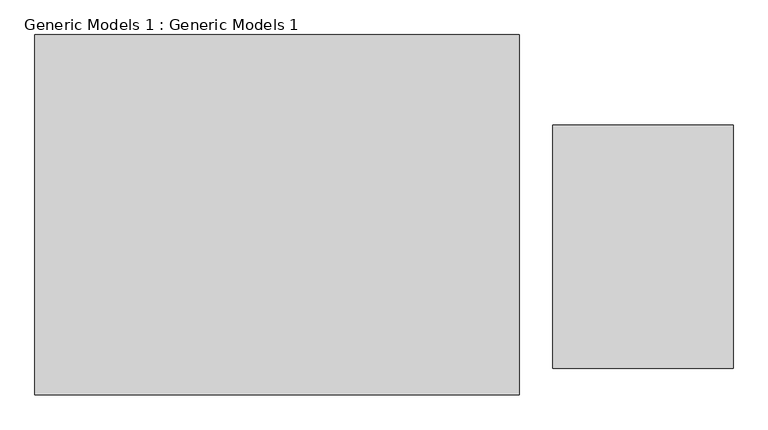
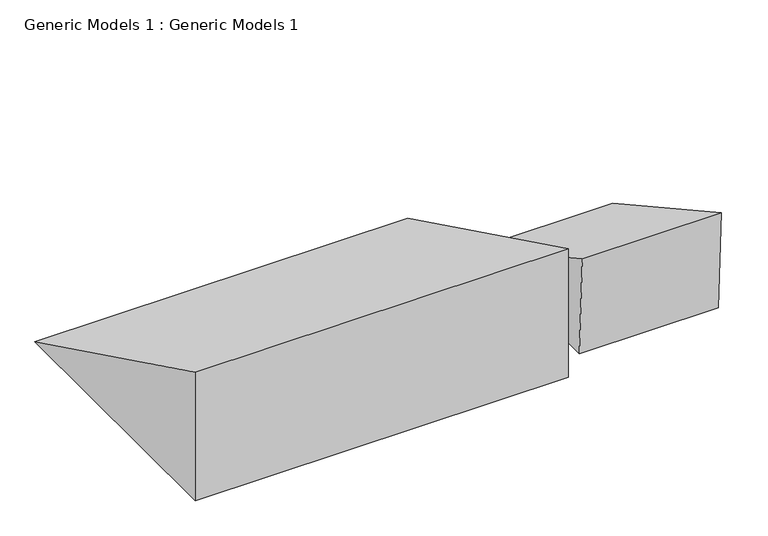
"""IFC4 building model written with IfcOpenShell, lengths in millimetres: proxy geometry, Generic Models 1 : Generic Models 1."""

from ifc_helpers import new_model, si_unit, frame, origin, place, context, project, spatial, polyline, outline, extrude, source, transform, mapped, element, save


def generic_models_1_generic_models_1_986dd2cf(model_context):
    return source(origin(), model_context, "Body", "SweptSolid", [
        extrude(outline(polyline([(-1395.5257947, -3200.4), (-2995.7257947, -3200.4), (-3043.5817931, -2287.2531534), (-1395.5257947, -3200.4)])), frame((-20052.0963079, 0.0, 0.0), z_axis=(1.0, 0.0, 0.0), x_axis=(0.0, 1.0, 0.0)), (0.0, 0.0, 1.0), 1219.2),
        extrude(outline(polyline([(-3224.3257947, -3200.4), (-3224.3257947, -2006.6), (-785.9257947, -3200.4), (-3224.3257947, -3200.4)])), frame((-23557.2963079, 0.0, 0.0), z_axis=(1.0, 0.0, 0.0), x_axis=(0.0, 1.0, 0.0)), (0.0, 0.0, 1.0), 3276.6),
    ])


if __name__ == "__main__":
    model = new_model("IFC4")
    model_context = context("Model", 3, world=origin())
    ifc_project = project(units=[si_unit("LENGTHUNIT", "METRE", prefix="MILLI")], contexts=[model_context])
    site = spatial("IfcSite", under=ifc_project)
    building = spatial("IfcBuilding", under=site)
    placement = place(None, origin())
    generic_models_1_generic_models_1_shape = generic_models_1_generic_models_1_986dd2cf(model_context)
    element("IfcBuildingElementProxy", 1, Name="Generic Models 1 : Generic Models 1", ObjectType="Generic Models 1 : Generic Models 1", at=placement, inside=building, context=model_context, shape_type="MappedRepresentation", body=[
        mapped(generic_models_1_generic_models_1_shape, transform((0.0, 0.0, 0.0), x_axis=(1.0, 0.0, 0.0), y_axis=(0.0, 1.0, 0.0), z_axis=(0.0, 0.0, 1.0))),
    ])
    save(model, "model.ifc")
